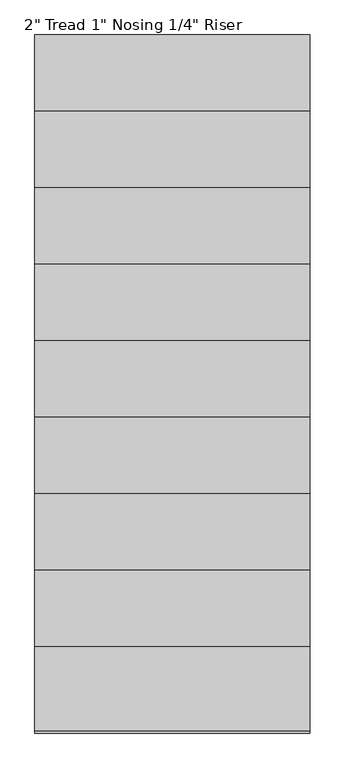
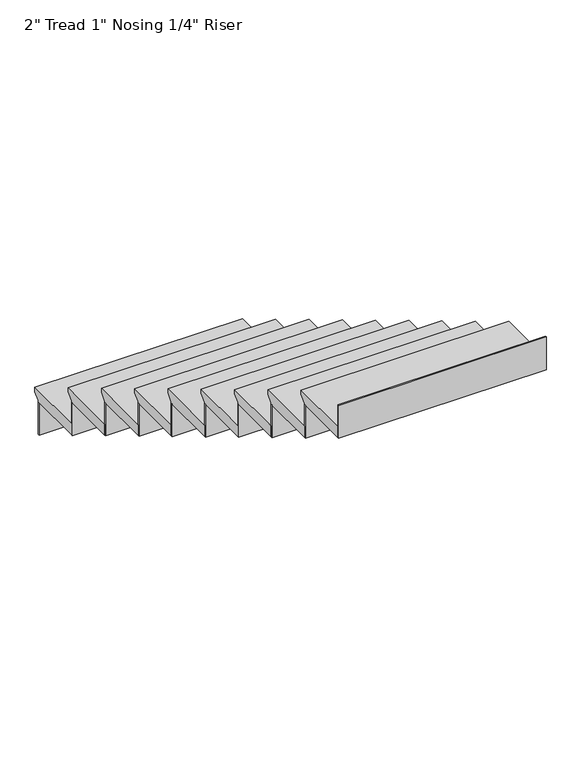
"""IFC4 building model written with IfcOpenShell, lengths in millimetres: stair flight geometry."""

from ifc_helpers import new_model, si_unit, frame, origin, place, context, project, spatial, polyline, outline, extrude, source, transform, mapped, element, save


def stair_flight_0e2f1c24(model_context):
    return source(origin(), model_context, "Body", "SweptSolid", [
        extrude(outline(polyline([(-2919.1227897, 1676.4), (-2639.7227897, 1676.4), (-2639.7227897, 1657.35), (-2665.1227897, 1631.95), (-2665.1227897, 1625.6), (-2919.1227897, 1625.6), (-2919.1227897, 1676.4)])), frame((-9500.8771954, 0.0, 0.0), z_axis=(1.0, 0.0, 0.0), x_axis=(0.0, 1.0, 0.0)), (0.0, 0.0, 1.0), 914.4),
        extrude(outline(polyline([(-9500.8771954, -2671.4727897), (-9500.8771954, -2665.1227897), (-8586.4771954, -2665.1227897), (-8586.4771954, -2671.4727897), (-9500.8771954, -2671.4727897)])), frame((0.0, 0.0, 1473.2), z_axis=(0.0, 0.0, 1.0), x_axis=(1.0, 0.0, 0.0)), (0.0, 0.0, 1.0), 152.4),
        extrude(outline(polyline([(-9500.8771954, -2925.4727897), (-9500.8771954, -2919.1227897), (-8586.4771954, -2919.1227897), (-8586.4771954, -2925.4727897), (-9500.8771954, -2925.4727897)])), frame((0.0, 0.0, 1625.6), z_axis=(0.0, 0.0, 1.0), x_axis=(1.0, 0.0, 0.0)), (0.0, 0.0, 1.0), 152.4),
        extrude(outline(polyline([(-3173.1227897, 1828.8), (-2893.7227897, 1828.8), (-2893.7227897, 1809.75), (-2919.1227897, 1784.35), (-2919.1227897, 1778.0), (-3173.1227897, 1778.0), (-3173.1227897, 1828.8)])), frame((-9500.8771954, 0.0, 0.0), z_axis=(1.0, 0.0, 0.0), x_axis=(0.0, 1.0, 0.0)), (0.0, 0.0, 1.0), 914.4),
        extrude(outline(polyline([(-9500.8771954, -3179.4727897), (-9500.8771954, -3173.1227897), (-8586.4771954, -3173.1227897), (-8586.4771954, -3179.4727897), (-9500.8771954, -3179.4727897)])), frame((0.0, 0.0, 1778.0), z_axis=(0.0, 0.0, 1.0), x_axis=(1.0, 0.0, 0.0)), (0.0, 0.0, 1.0), 152.4),
        extrude(outline(polyline([(-3427.1227897, 1981.2), (-3147.7227897, 1981.2), (-3147.7227897, 1962.15), (-3173.1227897, 1936.75), (-3173.1227897, 1930.4), (-3427.1227897, 1930.4), (-3427.1227897, 1981.2)])), frame((-9500.8771954, 0.0, 0.0), z_axis=(1.0, 0.0, 0.0), x_axis=(0.0, 1.0, 0.0)), (0.0, 0.0, 1.0), 914.4),
        extrude(outline(polyline([(-9500.8771954, -3433.4727897), (-9500.8771954, -3427.1227897), (-8586.4771954, -3427.1227897), (-8586.4771954, -3433.4727897), (-9500.8771954, -3433.4727897)])), frame((0.0, 0.0, 1930.4), z_axis=(0.0, 0.0, 1.0), x_axis=(1.0, 0.0, 0.0)), (0.0, 0.0, 1.0), 152.4),
        extrude(outline(polyline([(-3681.1227897, 2133.6), (-3401.7227897, 2133.6), (-3401.7227897, 2114.55), (-3427.1227897, 2089.15), (-3427.1227897, 2082.8), (-3681.1227897, 2082.8), (-3681.1227897, 2133.6)])), frame((-9500.8771954, 0.0, 0.0), z_axis=(1.0, 0.0, 0.0), x_axis=(0.0, 1.0, 0.0)), (0.0, 0.0, 1.0), 914.4),
        extrude(outline(polyline([(-9500.8771954, -3687.4727897), (-9500.8771954, -3681.1227897), (-8586.4771954, -3681.1227897), (-8586.4771954, -3687.4727897), (-9500.8771954, -3687.4727897)])), frame((0.0, 0.0, 2082.8), z_axis=(0.0, 0.0, 1.0), x_axis=(1.0, 0.0, 0.0)), (0.0, 0.0, 1.0), 152.4),
        extrude(outline(polyline([(-3935.1227897, 2286.0), (-3655.7227897, 2286.0), (-3655.7227897, 2266.95), (-3681.1227897, 2241.55), (-3681.1227897, 2235.2), (-3935.1227897, 2235.2), (-3935.1227897, 2286.0)])), frame((-9500.8771954, 0.0, 0.0), z_axis=(1.0, 0.0, 0.0), x_axis=(0.0, 1.0, 0.0)), (0.0, 0.0, 1.0), 914.4),
        extrude(outline(polyline([(-9500.8771954, -3941.4727897), (-9500.8771954, -3935.1227897), (-8586.4771954, -3935.1227897), (-8586.4771954, -3941.4727897), (-9500.8771954, -3941.4727897)])), frame((0.0, 0.0, 2235.2), z_axis=(0.0, 0.0, 1.0), x_axis=(1.0, 0.0, 0.0)), (0.0, 0.0, 1.0), 152.4),
        extrude(outline(polyline([(-4189.1227897, 2438.4), (-3909.7227897, 2438.4), (-3909.7227897, 2419.35), (-3935.1227897, 2393.95), (-3935.1227897, 2387.6), (-4189.1227897, 2387.6), (-4189.1227897, 2438.4)])), frame((-9500.8771954, 0.0, 0.0), z_axis=(1.0, 0.0, 0.0), x_axis=(0.0, 1.0, 0.0)), (0.0, 0.0, 1.0), 914.4),
        extrude(outline(polyline([(-9500.8771954, -4195.4727897), (-9500.8771954, -4189.1227897), (-8586.4771954, -4189.1227897), (-8586.4771954, -4195.4727897), (-9500.8771954, -4195.4727897)])), frame((0.0, 0.0, 2387.6), z_axis=(0.0, 0.0, 1.0), x_axis=(1.0, 0.0, 0.0)), (0.0, 0.0, 1.0), 152.4),
        extrude(outline(polyline([(-4443.1227897, 2590.8), (-4163.7227897, 2590.8), (-4163.7227897, 2571.75), (-4189.1227897, 2546.35), (-4189.1227897, 2540.0), (-4443.1227897, 2540.0), (-4443.1227897, 2590.8)])), frame((-9500.8771954, 0.0, 0.0), z_axis=(1.0, 0.0, 0.0), x_axis=(0.0, 1.0, 0.0)), (0.0, 0.0, 1.0), 914.4),
        extrude(outline(polyline([(-9500.8771954, -4449.4727897), (-9500.8771954, -4443.1227897), (-8586.4771954, -4443.1227897), (-8586.4771954, -4449.4727897), (-9500.8771954, -4449.4727897)])), frame((0.0, 0.0, 2540.0), z_axis=(0.0, 0.0, 1.0), x_axis=(1.0, 0.0, 0.0)), (0.0, 0.0, 1.0), 152.4),
        extrude(outline(polyline([(-4697.1227897, 2743.2), (-4417.7227897, 2743.2), (-4417.7227897, 2724.15), (-4443.1227897, 2698.75), (-4443.1227897, 2692.4), (-4697.1227897, 2692.4), (-4697.1227897, 2743.2)])), frame((-9500.8771954, 0.0, 0.0), z_axis=(1.0, 0.0, 0.0), x_axis=(0.0, 1.0, 0.0)), (0.0, 0.0, 1.0), 914.4),
        extrude(outline(polyline([(-9500.8771954, -4703.4727897), (-9500.8771954, -4697.1227897), (-8586.4771954, -4697.1227897), (-8586.4771954, -4703.4727897), (-9500.8771954, -4703.4727897)])), frame((0.0, 0.0, 2692.4), z_axis=(0.0, 0.0, 1.0), x_axis=(1.0, 0.0, 0.0)), (0.0, 0.0, 1.0), 152.4),
        extrude(outline(polyline([(-9500.8771954, -4957.4727897), (-9500.8771954, -4951.1227897), (-8586.4771954, -4951.1227897), (-8586.4771954, -4957.4727897), (-9500.8771954, -4957.4727897)])), frame((0.0, 0.0, 2844.8), z_axis=(0.0, 0.0, 1.0), x_axis=(1.0, 0.0, 0.0)), (0.0, 0.0, 1.0), 152.4),
        extrude(outline(polyline([(-4951.1227897, 2895.6), (-4671.7227897, 2895.6), (-4671.7227897, 2876.55), (-4697.1227897, 2851.15), (-4697.1227897, 2844.8), (-4951.1227897, 2844.8), (-4951.1227897, 2895.6)])), frame((-9500.8771954, 0.0, 0.0), z_axis=(1.0, 0.0, 0.0), x_axis=(0.0, 1.0, 0.0)), (0.0, 0.0, 1.0), 914.4),
    ])


if __name__ == "__main__":
    model = new_model("IFC4")
    model_context = context("Model", 3, world=origin())
    ifc_project = project(units=[si_unit("LENGTHUNIT", "METRE", prefix="MILLI")], contexts=[model_context])
    site = spatial("IfcSite", under=ifc_project)
    building = spatial("IfcBuilding", under=site)
    placement = place(None, origin())
    stair_flight_shape = stair_flight_0e2f1c24(model_context)
    element("IfcStairFlight", 1, ObjectType="2\" Tread 1\" Nosing 1/4\" Riser", at=placement, inside=building, context=model_context, shape_type="MappedRepresentation", body=[
        mapped(stair_flight_shape, transform((0.0, 0.0, 0.0), x_axis=(1.0, 0.0, 0.0), y_axis=(0.0, 1.0, 0.0), z_axis=(0.0, 0.0, 1.0))),
    ])
    save(model, "model.ifc")

# Revit data of these elements
# Element 1 (IfcStairFlight, "2\" Tread 1\" Nosing 1/4\" Riser")
#   Materials on its faces: "Porcelain, Linen"
# Materials
#   "Porcelain, Linen": class "Ceramic", colour RGB 249 239 230, transparency 0, Description = "Porcelain, linen", Cost = 0
